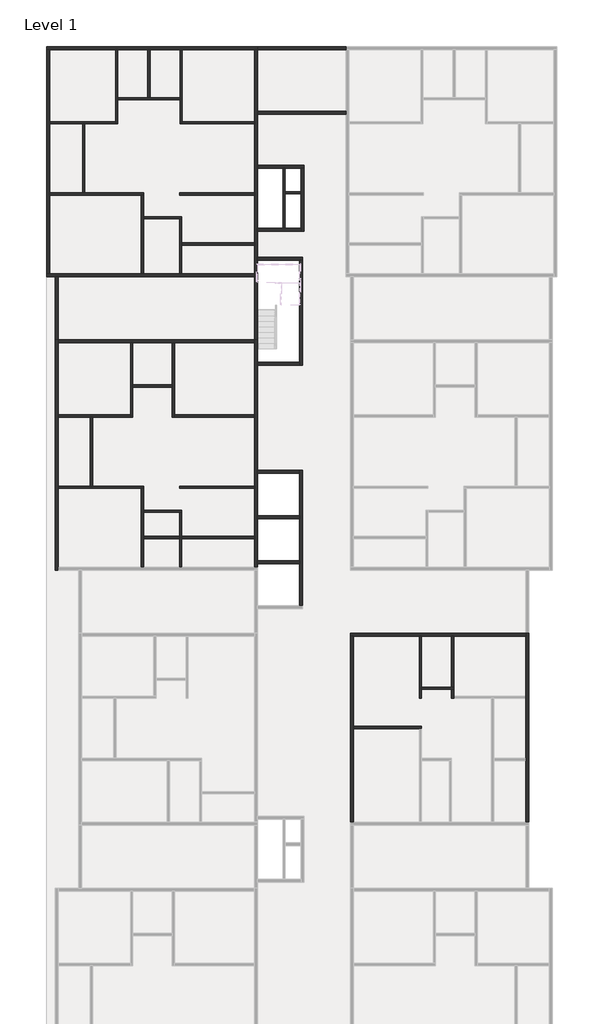
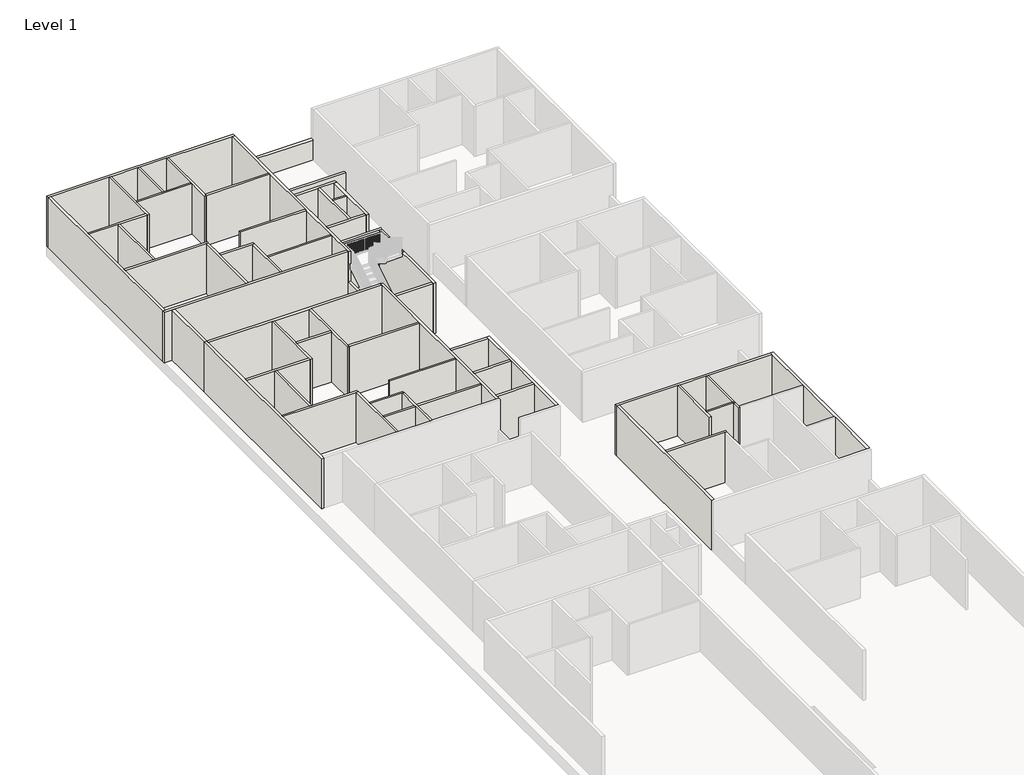
# One storey, part 3 of 8: 57 walls.
"""IFC4 building model written with IfcOpenShell, lengths in millimetres."""

from ifc_helpers import new_model, si_unit, frame, origin, place, context, project, spatial, polyline, outline, extrude, faceted_brep, element, save

model = new_model("IFC4")

# Units and contexts
model_context = context("Model", 3, world=origin())
ifc_project = project(units=[si_unit("LENGTHUNIT", "METRE", prefix="MILLI")], contexts=[model_context])

# Site, building, storey
site = spatial("IfcSite", under=ifc_project)
building = spatial("IfcBuilding", under=site)
storey = spatial("IfcBuildingStorey", under=building, Name="Level 1", Elevation=25234.6172466)

# Walls
placement = place(None, origin())
element("IfcWall", 1, ObjectType="4.5\"", at=placement, inside=storey, context=model_context, shape_type="Brep", body=[
    faceted_brep([(-10818.3415084, 35031.1216096, 25234.6172466), (-10818.3415084, 31373.5216096, 25234.6172466), (-10818.3415084, 31259.2216096, 25234.6172466), (-10818.3415084, 31259.2216096, 28282.6172466), (-10818.3415084, 31373.5216096, 28282.6172466), (-10818.3415084, 35031.1216096, 28282.6172466), (-10704.0415084, 35031.1216096, 25234.6172466), (-10704.0415084, 35031.1216096, 28282.6172466), (-10704.0415084, 32592.7216096, 28282.6172466), (-10704.0415084, 32478.4216096, 28282.6172466), (-10704.0415084, 31259.2216096, 28282.6172466), (-10704.0415084, 31259.2216096, 25234.6172466), (-10704.0415084, 32478.4216096, 25234.6172466), (-10704.0415084, 32592.7216096, 25234.6172466)], [[[0, 1, 2, 3, 4, 5]], [[6, 7, 8, 9, 10, 11, 12, 13]], [[2, 1, 0, 6, 13, 12, 11]], [[0, 5, 7, 6]], [[3, 2, 11, 10]], [[5, 4, 3, 10, 9, 8, 7]]]),
])
element("IfcWall", 2, ObjectType="4.5\"", at=placement, inside=storey, context=model_context, shape_type="Brep", body=[
    faceted_brep([(-10818.3415084, 31373.5216096, 25234.6172466), (-14171.1415084, 31373.5216096, 25234.6172466), (-14171.1415084, 31373.5216096, 28282.6172466), (-10818.3415084, 31373.5216096, 28282.6172466), (-10818.3415084, 31259.2216096, 25234.6172466), (-10818.3415084, 31259.2216096, 28282.6172466), (-12380.4415084, 31259.2216096, 28282.6172466), (-12494.7415084, 31259.2216096, 28282.6172466), (-14171.1415084, 31259.2216096, 28282.6172466), (-14171.1415084, 31259.2216096, 25234.6172466), (-12494.7415084, 31259.2216096, 25234.6172466), (-12380.4415084, 31259.2216096, 25234.6172466)], [[[0, 1, 2, 3]], [[4, 5, 6, 7, 8, 9, 10, 11]], [[1, 0, 4, 11, 10, 9]], [[0, 3, 5, 4]], [[2, 1, 9, 8]], [[3, 2, 8, 7, 6, 5]]]),
])
element("IfcWall", 3, ObjectType="4.5\"", at=placement, inside=storey, context=model_context, shape_type="SweptSolid", body=[
    extrude(outline(polyline([(-12494.7415084, 27754.0216096), (-12494.7415084, 31259.2216096), (-12380.4415084, 31259.2216096), (-12380.4415084, 27754.0216096), (-12494.7415084, 27754.0216096)])), frame((0.0, 0.0, 25234.6172466), z_axis=(0.0, 0.0, 1.0), x_axis=(1.0, 0.0, 0.0)), (0.0, 0.0, 1.0), 3048.0),
])
element("IfcWall", 4, ObjectType="4.5\"", at=placement, inside=storey, context=model_context, shape_type="Brep", body=[
    faceted_brep([(-14171.1415084, 27639.7216096, 25234.6172466), (-9510.2415084, 27639.7216096, 25234.6172466), (-9395.9415084, 27639.7216096, 25234.6172466), (-9395.9415084, 27639.7216096, 28282.6172466), (-9510.2415084, 27639.7216096, 28282.6172466), (-14171.1415084, 27639.7216096, 28282.6172466), (-14171.1415084, 27754.0216096, 25234.6172466), (-14171.1415084, 27754.0216096, 28282.6172466), (-12494.7415084, 27754.0216096, 28282.6172466), (-12380.4415084, 27754.0216096, 28282.6172466), (-9395.9415084, 27754.0216096, 28282.6172466), (-9395.9415084, 27754.0216096, 25234.6172466), (-12380.4415084, 27754.0216096, 25234.6172466), (-12494.7415084, 27754.0216096, 25234.6172466)], [[[0, 1, 2, 3, 4, 5]], [[6, 7, 8, 9, 10, 11, 12, 13]], [[2, 1, 0, 6, 13, 12, 11]], [[0, 5, 7, 6]], [[3, 2, 11, 10]], [[5, 4, 3, 10, 9, 8, 7]]]),
])
element("IfcWall", 5, ObjectType="4.5\"", at=placement, inside=storey, context=model_context, shape_type="Brep", body=[
    faceted_brep([(-9510.2415084, 27639.7216096, 25234.6172466), (-9510.2415084, 23651.9216096, 25234.6172466), (-9510.2415084, 23651.9216096, 28282.6172466), (-9510.2415084, 27639.7216096, 28282.6172466), (-9395.9415084, 27639.7216096, 25234.6172466), (-9395.9415084, 27639.7216096, 28282.6172466), (-9395.9415084, 26547.5216096, 28282.6172466), (-9395.9415084, 26433.2216096, 28282.6172466), (-9395.9415084, 23651.9216096, 28282.6172466), (-9395.9415084, 23651.9216096, 25234.6172466), (-9395.9415084, 26433.2216096, 25234.6172466), (-9395.9415084, 26547.5216096, 25234.6172466)], [[[0, 1, 2, 3]], [[4, 5, 6, 7, 8, 9, 10, 11]], [[1, 0, 4, 11, 10, 9]], [[0, 3, 5, 4]], [[2, 1, 9, 8]], [[3, 2, 8, 7, 6, 5]]]),
])
element("IfcWall", 6, ObjectType="4.5\"", at=placement, inside=storey, context=model_context, shape_type="Brep", body=[
    faceted_brep([(-9395.9415084, 26433.2216096, 25234.6172466), (-7567.1415084, 26433.2216096, 25234.6172466), (-7452.8415084, 26433.2216096, 25234.6172466), (-7452.8415084, 26433.2216096, 28282.6172466), (-7567.1415084, 26433.2216096, 28282.6172466), (-9395.9415084, 26433.2216096, 28282.6172466), (-9395.9415084, 26547.5216096, 25234.6172466), (-9395.9415084, 26547.5216096, 28282.6172466), (-7452.8415084, 26547.5216096, 28282.6172466), (-7452.8415084, 26547.5216096, 25234.6172466)], [[[0, 1, 2, 3, 4, 5]], [[6, 7, 8, 9]], [[2, 1, 0, 6, 9]], [[0, 5, 7, 6]], [[3, 2, 9, 8]], [[5, 4, 3, 8, 7]]]),
])
element("IfcWall", 7, ObjectType="4.5\"", at=placement, inside=storey, context=model_context, shape_type="Brep", body=[
    faceted_brep([(-7567.1415084, 26433.2216096, 25234.6172466), (-7567.1415084, 23651.9216096, 25234.6172466), (-7567.1415084, 23651.9216096, 28282.6172466), (-7567.1415084, 26433.2216096, 28282.6172466), (-7452.8415084, 26433.2216096, 25234.6172466), (-7452.8415084, 26433.2216096, 28282.6172466), (-7452.8415084, 25214.0216096, 28282.6172466), (-7452.8415084, 25099.7216096, 28282.6172466), (-7452.8415084, 23651.9216096, 28282.6172466), (-7452.8415084, 23651.9216096, 25234.6172466), (-7452.8415084, 25099.7216096, 25234.6172466), (-7452.8415084, 25214.0216096, 25234.6172466)], [[[0, 1, 2, 3]], [[4, 5, 6, 7, 8, 9, 10, 11]], [[1, 0, 4, 11, 10, 9]], [[0, 3, 5, 4]], [[2, 1, 9, 8]], [[3, 2, 8, 7, 6, 5]]]),
])
element("IfcWall", 8, ObjectType="4.5\"", at=placement, inside=storey, context=model_context, shape_type="SweptSolid", body=[
    extrude(outline(polyline([(-7452.8415084, 25214.0216096), (-3769.8415084, 25214.0216096), (-3769.8415084, 25099.7216096), (-7452.8415084, 25099.7216096), (-7452.8415084, 25214.0216096)])), frame((0.0, 0.0, 25234.6172466), z_axis=(0.0, 0.0, 1.0), x_axis=(1.0, 0.0, 0.0)), (0.0, 0.0, 1.0), 3048.0),
])
element("IfcWall", 9, ObjectType="4.5\"", at=placement, inside=storey, context=model_context, shape_type="SweptSolid", body=[
    extrude(outline(polyline([(-3769.8415084, 27639.7216096), (-7567.1415084, 27639.7216096), (-7567.1415084, 27754.0216096), (-3769.8415084, 27754.0216096), (-3769.8415084, 27639.7216096)])), frame((0.0, 0.0, 25234.6172466), z_axis=(0.0, 0.0, 1.0), x_axis=(1.0, 0.0, 0.0)), (0.0, 0.0, 1.0), 3048.0),
])
element("IfcWall", 10, ObjectType="4.5\"", at=placement, inside=storey, context=model_context, shape_type="Brep", body=[
    faceted_brep([(-10704.0415084, 32478.4216096, 25234.6172466), (-7541.7415084, 32478.4216096, 25234.6172466), (-7541.7415084, 32478.4216096, 28282.6172466), (-10704.0415084, 32478.4216096, 28282.6172466), (-10704.0415084, 32592.7216096, 25234.6172466), (-10704.0415084, 32592.7216096, 28282.6172466), (-9180.0415084, 32592.7216096, 28282.6172466), (-9065.7415084, 32592.7216096, 28282.6172466), (-7541.7415084, 32592.7216096, 28282.6172466), (-7541.7415084, 32592.7216096, 25234.6172466), (-9065.7415084, 32592.7216096, 25234.6172466), (-9180.0415084, 32592.7216096, 25234.6172466)], [[[0, 1, 2, 3]], [[4, 5, 6, 7, 8, 9, 10, 11]], [[1, 0, 4, 11, 10, 9]], [[0, 3, 5, 4]], [[2, 1, 9, 8]], [[3, 2, 8, 7, 6, 5]]]),
])
element("IfcWall", 11, ObjectType="4.5\"", at=placement, inside=storey, context=model_context, shape_type="SweptSolid", body=[
    extrude(outline(polyline([(-9180.0415084, 32592.7216096), (-9180.0415084, 35031.1216096), (-9065.7415084, 35031.1216096), (-9065.7415084, 32592.7216096), (-9180.0415084, 32592.7216096)])), frame((0.0, 0.0, 25234.6172466), z_axis=(0.0, 0.0, 1.0), x_axis=(1.0, 0.0, 0.0)), (0.0, 0.0, 1.0), 3048.0),
])
element("IfcWall", 12, ObjectType="4.5\"", at=placement, inside=storey, context=model_context, shape_type="Brep", body=[
    faceted_brep([(-7541.7415084, 35031.1216096, 25234.6172466), (-7541.7415084, 32592.7216096, 25234.6172466), (-7541.7415084, 32478.4216096, 25234.6172466), (-7541.7415084, 31259.2216096, 25234.6172466), (-7541.7415084, 31259.2216096, 28282.6172466), (-7541.7415084, 32478.4216096, 28282.6172466), (-7541.7415084, 32592.7216096, 28282.6172466), (-7541.7415084, 35031.1216096, 28282.6172466), (-7427.4415084, 35031.1216096, 25234.6172466), (-7427.4415084, 35031.1216096, 28282.6172466), (-7427.4415084, 31373.5216096, 28282.6172466), (-7427.4415084, 31259.2216096, 28282.6172466), (-7427.4415084, 31259.2216096, 25234.6172466), (-7427.4415084, 31373.5216096, 25234.6172466)], [[[0, 1, 2, 3, 4, 5, 6, 7]], [[8, 9, 10, 11, 12, 13]], [[3, 2, 1, 0, 8, 13, 12]], [[0, 7, 9, 8]], [[4, 3, 12, 11]], [[7, 6, 5, 4, 11, 10, 9]]]),
])
element("IfcWall", 13, ObjectType="4.5\"", at=placement, inside=storey, context=model_context, shape_type="SweptSolid", body=[
    extrude(outline(polyline([(-3769.8415084, 31259.2216096), (-7427.4415084, 31259.2216096), (-7427.4415084, 31373.5216096), (-3769.8415084, 31373.5216096), (-3769.8415084, 31259.2216096)])), frame((0.0, 0.0, 25234.6172466), z_axis=(0.0, 0.0, 1.0), x_axis=(1.0, 0.0, 0.0)), (0.0, 0.0, 1.0), 3048.0),
])
element("IfcWall", 14, ObjectType="4.5\"", at=placement, inside=storey, context=model_context, shape_type="Brep", body=[
    faceted_brep([(-10061.4044854, 20146.7216096, 25234.6172466), (-10061.4044854, 16489.1216096, 25234.6172466), (-10061.4044854, 16374.8216096, 25234.6172466), (-10061.4044854, 16374.8216096, 28282.6172466), (-10061.4044854, 16489.1216096, 28282.6172466), (-10061.4044854, 20146.7216096, 28282.6172466), (-9947.1044854, 20146.7216096, 25234.6172466), (-9947.1044854, 20146.7216096, 28282.6172466), (-9947.1044854, 18013.1216096, 28282.6172466), (-9947.1044854, 17898.8216096, 28282.6172466), (-9947.1044854, 16374.8216096, 28282.6172466), (-9947.1044854, 16374.8216096, 25234.6172466), (-9947.1044854, 17898.8216096, 25234.6172466), (-9947.1044854, 18013.1216096, 25234.6172466)], [[[0, 1, 2, 3, 4, 5]], [[6, 7, 8, 9, 10, 11, 12, 13]], [[2, 1, 0, 6, 13, 12, 11]], [[0, 5, 7, 6]], [[3, 2, 11, 10]], [[5, 4, 3, 10, 9, 8, 7]]]),
])
element("IfcWall", 15, ObjectType="4.5\"", at=placement, inside=storey, context=model_context, shape_type="Brep", body=[
    faceted_brep([(-10061.4044854, 16489.1216096, 25234.6172466), (-13719.0044854, 16489.1216096, 25234.6172466), (-13719.0044854, 16489.1216096, 28282.6172466), (-10061.4044854, 16489.1216096, 28282.6172466), (-10061.4044854, 16374.8216096, 25234.6172466), (-10061.4044854, 16374.8216096, 28282.6172466), (-11980.3915084, 16374.8216096, 28282.6172466), (-12094.6915084, 16374.8216096, 28282.6172466), (-13719.0044854, 16374.8216096, 28282.6172466), (-13719.0044854, 16374.8216096, 25234.6172466), (-12094.6915084, 16374.8216096, 25234.6172466), (-11980.3915084, 16374.8216096, 25234.6172466)], [[[0, 1, 2, 3]], [[4, 5, 6, 7, 8, 9, 10, 11]], [[1, 0, 4, 11, 10, 9]], [[0, 3, 5, 4]], [[2, 1, 9, 8]], [[3, 2, 8, 7, 6, 5]]]),
])
element("IfcWall", 16, ObjectType="4.5\"", at=placement, inside=storey, context=model_context, shape_type="SweptSolid", body=[
    extrude(outline(polyline([(-7940.5044854, 17898.8216096), (-9947.1044854, 17898.8216096), (-9947.1044854, 18013.1216096), (-7940.5044854, 18013.1216096), (-7940.5044854, 17898.8216096)])), frame((0.0, 0.0, 25234.6172466), z_axis=(0.0, 0.0, 1.0), x_axis=(1.0, 0.0, 0.0)), (0.0, 0.0, 1.0), 3048.0),
])
element("IfcWall", 17, ObjectType="4.5\"", at=placement, inside=storey, context=model_context, shape_type="Brep", body=[
    faceted_brep([(-7940.5044854, 20146.7216096, 25234.6172466), (-7940.5044854, 18013.1216096, 25234.6172466), (-7940.5044854, 17898.8216096, 25234.6172466), (-7940.5044854, 16374.8216096, 25234.6172466), (-7940.5044854, 16374.8216096, 28282.6172466), (-7940.5044854, 17898.8216096, 28282.6172466), (-7940.5044854, 18013.1216096, 28282.6172466), (-7940.5044854, 20146.7216096, 28282.6172466), (-7826.2044854, 20146.7216096, 25234.6172466), (-7826.2044854, 20146.7216096, 28282.6172466), (-7826.2044854, 16489.1216096, 28282.6172466), (-7826.2044854, 16374.8216096, 28282.6172466), (-7826.2044854, 16374.8216096, 25234.6172466), (-7826.2044854, 16489.1216096, 25234.6172466)], [[[0, 1, 2, 3, 4, 5, 6, 7]], [[8, 9, 10, 11, 12, 13]], [[3, 2, 1, 0, 8, 13, 12]], [[0, 7, 9, 8]], [[4, 3, 12, 11]], [[7, 6, 5, 4, 11, 10, 9]]]),
])
element("IfcWall", 18, ObjectType="4.5\"", at=placement, inside=storey, context=model_context, shape_type="SweptSolid", body=[
    extrude(outline(polyline([(-3769.8415084, 16374.8216096), (-7826.2044854, 16374.8216096), (-7826.2044854, 16489.1216096), (-3769.8415084, 16489.1216096), (-3769.8415084, 16374.8216096)])), frame((0.0, 0.0, 25234.6172466), z_axis=(0.0, 0.0, 1.0), x_axis=(1.0, 0.0, 0.0)), (0.0, 0.0, 1.0), 3048.0),
])
element("IfcWall", 19, ObjectType="4.5\"", at=placement, inside=storey, context=model_context, shape_type="SweptSolid", body=[
    extrude(outline(polyline([(-12094.6915084, 12869.6216096), (-12094.6915084, 16374.8216096), (-11980.3915084, 16374.8216096), (-11980.3915084, 12869.6216096), (-12094.6915084, 12869.6216096)])), frame((0.0, 0.0, 25234.6172466), z_axis=(0.0, 0.0, 1.0), x_axis=(1.0, 0.0, 0.0)), (0.0, 0.0, 1.0), 3048.0),
])
element("IfcWall", 20, ObjectType="4.5\"", at=placement, inside=storey, context=model_context, shape_type="Brep", body=[
    faceted_brep([(-13719.0044854, 12755.3216096, 25234.6172466), (-9510.2415084, 12755.3216096, 25234.6172466), (-9395.9415084, 12755.3216096, 25234.6172466), (-9395.9415084, 12755.3216096, 28282.6172466), (-9510.2415084, 12755.3216096, 28282.6172466), (-13719.0044854, 12755.3216096, 28282.6172466), (-13719.0044854, 12869.6216096, 25234.6172466), (-13719.0044854, 12869.6216096, 28282.6172466), (-12094.6915084, 12869.6216096, 28282.6172466), (-11980.3915084, 12869.6216096, 28282.6172466), (-9395.9415084, 12869.6216096, 28282.6172466), (-9395.9415084, 12869.6216096, 25234.6172466), (-11980.3915084, 12869.6216096, 25234.6172466), (-12094.6915084, 12869.6216096, 25234.6172466)], [[[0, 1, 2, 3, 4, 5]], [[6, 7, 8, 9, 10, 11, 12, 13]], [[2, 1, 0, 6, 13, 12, 11]], [[0, 5, 7, 6]], [[3, 2, 11, 10]], [[5, 4, 3, 10, 9, 8, 7]]]),
])
element("IfcWall", 21, ObjectType="4.5\"", at=placement, inside=storey, context=model_context, shape_type="Brep", body=[
    faceted_brep([(-9510.2415084, 12755.3216096, 25234.6172466), (-9510.2415084, 8767.5216096, 25234.6172466), (-9510.2415084, 8767.5216096, 28282.6172466), (-9510.2415084, 12755.3216096, 28282.6172466), (-9395.9415084, 12755.3216096, 25234.6172466), (-9395.9415084, 12755.3216096, 28282.6172466), (-9395.9415084, 11663.1216096, 28282.6172466), (-9395.9415084, 11548.8216096, 28282.6172466), (-9395.9415084, 10329.6216096, 28282.6172466), (-9395.9415084, 10215.3216096, 28282.6172466), (-9395.9415084, 8767.5216096, 28282.6172466), (-9395.9415084, 8767.5216096, 25234.6172466), (-9395.9415084, 10215.3216096, 25234.6172466), (-9395.9415084, 10329.6216096, 25234.6172466), (-9395.9415084, 11548.8216096, 25234.6172466), (-9395.9415084, 11663.1216096, 25234.6172466)], [[[0, 1, 2, 3]], [[4, 5, 6, 7, 8, 9, 10, 11, 12, 13, 14, 15]], [[1, 0, 4, 15, 14, 13, 12, 11]], [[0, 3, 5, 4]], [[2, 1, 11, 10]], [[3, 2, 10, 9, 8, 7, 6, 5]]]),
])
element("IfcWall", 22, ObjectType="4.5\"", at=placement, inside=storey, context=model_context, shape_type="SweptSolid", body=[
    extrude(outline(polyline([(-7567.1415084, 10215.3216096), (-9395.9415084, 10215.3216096), (-9395.9415084, 10329.6216096), (-7567.1415084, 10329.6216096), (-7567.1415084, 10215.3216096)])), frame((0.0, 0.0, 25234.6172466), z_axis=(0.0, 0.0, 1.0), x_axis=(1.0, 0.0, 0.0)), (0.0, 0.0, 1.0), 3048.0),
])
element("IfcWall", 23, ObjectType="4.5\"", at=placement, inside=storey, context=model_context, shape_type="Brep", body=[
    faceted_brep([(-9395.9415084, 11548.8216096, 25234.6172466), (-7567.1415084, 11548.8216096, 25234.6172466), (-7452.8415084, 11548.8216096, 25234.6172466), (-7452.8415084, 11548.8216096, 28282.6172466), (-7567.1415084, 11548.8216096, 28282.6172466), (-9395.9415084, 11548.8216096, 28282.6172466), (-9395.9415084, 11663.1216096, 25234.6172466), (-9395.9415084, 11663.1216096, 28282.6172466), (-7452.8415084, 11663.1216096, 28282.6172466), (-7452.8415084, 11663.1216096, 25234.6172466)], [[[0, 1, 2, 3, 4, 5]], [[6, 7, 8, 9]], [[2, 1, 0, 6, 9]], [[0, 5, 7, 6]], [[3, 2, 9, 8]], [[5, 4, 3, 8, 7]]]),
])
element("IfcWall", 24, ObjectType="4.5\"", at=placement, inside=storey, context=model_context, shape_type="Brep", body=[
    faceted_brep([(-7567.1415084, 11548.8216096, 25234.6172466), (-7567.1415084, 10329.6216096, 25234.6172466), (-7567.1415084, 10215.3216096, 25234.6172466), (-7567.1415084, 8767.5216096, 25234.6172466), (-7567.1415084, 8767.5216096, 28282.6172466), (-7567.1415084, 10215.3216096, 28282.6172466), (-7567.1415084, 10329.6216096, 28282.6172466), (-7567.1415084, 11548.8216096, 28282.6172466), (-7452.8415084, 11548.8216096, 25234.6172466), (-7452.8415084, 11548.8216096, 28282.6172466), (-7452.8415084, 10329.6216096, 28282.6172466), (-7452.8415084, 10215.3216096, 28282.6172466), (-7452.8415084, 8767.5216096, 28282.6172466), (-7452.8415084, 8767.5216096, 25234.6172466), (-7452.8415084, 10215.3216096, 25234.6172466), (-7452.8415084, 10329.6216096, 25234.6172466)], [[[0, 1, 2, 3, 4, 5, 6, 7]], [[8, 9, 10, 11, 12, 13, 14, 15]], [[3, 2, 1, 0, 8, 15, 14, 13]], [[0, 7, 9, 8]], [[4, 3, 13, 12]], [[7, 6, 5, 4, 12, 11, 10, 9]]]),
])
element("IfcWall", 25, ObjectType="4.5\"", at=placement, inside=storey, context=model_context, shape_type="SweptSolid", body=[
    extrude(outline(polyline([(-3769.8415084, 10215.3216096), (-7452.8415084, 10215.3216096), (-7452.8415084, 10329.6216096), (-3769.8415084, 10329.6216096), (-3769.8415084, 10215.3216096)])), frame((0.0, 0.0, 25234.6172466), z_axis=(0.0, 0.0, 1.0), x_axis=(1.0, 0.0, 0.0)), (0.0, 0.0, 1.0), 3048.0),
])
element("IfcWall", 26, ObjectType="4.5\"", at=placement, inside=storey, context=model_context, shape_type="SweptSolid", body=[
    extrude(outline(polyline([(-3769.8415084, 12755.3216096), (-7567.1415084, 12755.3216096), (-7567.1415084, 12869.6216096), (-3769.8415084, 12869.6216096), (-3769.8415084, 12755.3216096)])), frame((0.0, 0.0, 25234.6172466), z_axis=(0.0, 0.0, 1.0), x_axis=(1.0, 0.0, 0.0)), (0.0, 0.0, 1.0), 3048.0),
])
element("IfcWall", 27, ObjectType="4.5\"", at=placement, inside=storey, context=model_context, shape_type="Brep", body=[
    faceted_brep([(1259.3584916, 572.7745083, 25234.6172466), (4610.8714687, 572.7745083, 25234.6172466), (4725.1714687, 572.7745083, 25234.6172466), (4725.1714687, 572.7745083, 28282.6172466), (4610.8714687, 572.7745083, 28282.6172466), (1259.3584916, 572.7745083, 28282.6172466), (1259.3584916, 687.0745083, 25234.6172466), (1259.3584916, 687.0745083, 28282.6172466), (4725.1714687, 687.0745083, 28282.6172466), (4725.1714687, 687.0745083, 25234.6172466)], [[[0, 1, 2, 3, 4, 5]], [[6, 7, 8, 9]], [[2, 1, 0, 6, 9]], [[0, 5, 7, 6]], [[3, 2, 9, 8]], [[5, 4, 3, 8, 7]]]),
])
element("IfcWall", 28, ObjectType="4.5\"", at=placement, inside=storey, context=model_context, shape_type="Brep", body=[
    faceted_brep([(4610.8714687, 5262.3216096, 25234.6172466), (4610.8714687, 2100.0216096, 25234.6172466), (4610.8714687, 2100.0216096, 28282.6172466), (4610.8714687, 5262.3216096, 28282.6172466), (4725.1714687, 5262.3216096, 25234.6172466), (4725.1714687, 5262.3216096, 28282.6172466), (4725.1714687, 2671.5216096, 28282.6172466), (4725.1714687, 2557.2216096, 28282.6172466), (4725.1714687, 2100.0216096, 28282.6172466), (4725.1714687, 2100.0216096, 25234.6172466), (4725.1714687, 2557.2216096, 25234.6172466), (4725.1714687, 2671.5216096, 25234.6172466)], [[[0, 1, 2, 3]], [[4, 5, 6, 7, 8, 9, 10, 11]], [[1, 0, 4, 11, 10, 9]], [[2, 1, 9, 8]], [[0, 3, 5, 4]], [[3, 2, 8, 7, 6, 5]]]),
])
element("IfcWall", 29, ObjectType="4.5\"", at=placement, inside=storey, context=model_context, shape_type="Brep", body=[
    faceted_brep([(4725.1714687, 2557.2216096, 25234.6172466), (6249.1714687, 2557.2216096, 25234.6172466), (6363.4714687, 2557.2216096, 25234.6172466), (6363.4714687, 2557.2216096, 28282.6172466), (6249.1714687, 2557.2216096, 28282.6172466), (4725.1714687, 2557.2216096, 28282.6172466), (4725.1714687, 2671.5216096, 25234.6172466), (4725.1714687, 2671.5216096, 28282.6172466), (6249.1714687, 2671.5216096, 28282.6172466), (6363.4714687, 2671.5216096, 28282.6172466), (6363.4714687, 2671.5216096, 25234.6172466), (6249.1714687, 2671.5216096, 25234.6172466)], [[[0, 1, 2, 3, 4, 5]], [[6, 7, 8, 9, 10, 11]], [[2, 1, 0, 6, 11, 10]], [[0, 5, 7, 6]], [[3, 2, 10, 9]], [[5, 4, 3, 9, 8, 7]]]),
])
element("IfcWall", 30, ObjectType="4.5\"", at=placement, inside=storey, context=model_context, shape_type="SweptSolid", body=[
    extrude(outline(polyline([(6363.4714687, 5262.3216096), (6363.4714687, 2671.5216096), (6249.1714687, 2671.5216096), (6249.1714687, 5262.3216096), (6363.4714687, 5262.3216096)])), frame((0.0, 0.0, 25234.6172466), z_axis=(0.0, 0.0, 1.0), x_axis=(1.0, 0.0, 0.0)), (0.0, 0.0, 1.0), 3048.0),
])
element("IfcWall", 31, ObjectType="4.5\"", at=placement, inside=storey, context=model_context, shape_type="Brep", body=[
    faceted_brep([(6249.1714687, 2557.2216096, 25234.6172466), (6249.1714687, 2100.0216096, 25234.6172466), (6249.1714687, 2100.0216096, 28282.6172466), (6249.1714687, 2557.2216096, 28282.6172466), (6363.4714687, 2557.2216096, 25234.6172466), (6363.4714687, 2557.2216096, 28282.6172466), (6363.4714687, 2214.3216096, 28282.6172466), (6363.4714687, 2100.0216096, 28282.6172466), (6363.4714687, 2100.0216096, 25234.6172466), (6363.4714687, 2214.3216096, 25234.6172466)], [[[0, 1, 2, 3]], [[4, 5, 6, 7, 8, 9]], [[1, 0, 4, 9, 8]], [[0, 3, 5, 4]], [[2, 1, 8, 7]], [[3, 2, 7, 6, 5]]]),
])
element("IfcWall", 32, ObjectType="4.5\"", at=placement, inside=storey, context=model_context, shape_type="Brep", body=[
    faceted_brep([(-2321.9738684, 29000.0900967, 25234.6172466), (-2321.9738684, 25952.0900967, 25234.6172466), (-2321.9738684, 25952.0900967, 28282.6172466), (-2321.9738684, 29000.0900967, 28282.6172466), (-2207.6738684, 29000.0900967, 25234.6172466), (-2207.6738684, 29000.0900967, 28282.6172466), (-2207.6738684, 27820.8172885, 28282.6172466), (-2207.6738684, 27706.5172885, 28282.6172466), (-2207.6738684, 25952.0900967, 28282.6172466), (-2207.6738684, 25952.0900967, 25234.6172466), (-2207.6738684, 27706.5172885, 25234.6172466), (-2207.6738684, 27820.8172885, 25234.6172466)], [[[0, 1, 2, 3]], [[4, 5, 6, 7, 8, 9, 10, 11]], [[1, 0, 4, 11, 10, 9]], [[3, 2, 8, 7, 6, 5]], [[0, 3, 5, 4]], [[2, 1, 9, 8]]]),
])
element("IfcWall", 33, ObjectType="4.5\"", at=placement, inside=storey, context=model_context, shape_type="SweptSolid", body=[
    extrude(outline(polyline([(-2207.6738684, 27820.8172885), (-1407.6415084, 27820.8172885), (-1407.6415084, 27706.5172885), (-2207.6738684, 27706.5172885), (-2207.6738684, 27820.8172885)])), frame((0.0, 0.0, 25234.6172466), z_axis=(0.0, 0.0, 1.0), x_axis=(1.0, 0.0, 0.0)), (0.0, 0.0, 1.0), 3048.0),
])
element("IfcWall", 34, ObjectType="6\"", at=placement, inside=storey, context=model_context, shape_type="Brep", body=[
    faceted_brep([(-14323.5415084, 35031.1216096, 25234.6172466), (-14171.1415084, 35031.1216096, 25234.6172466), (-10818.3415084, 35031.1216096, 25234.6172466), (-10704.0415084, 35031.1216096, 25234.6172466), (-9180.0415084, 35031.1216096, 25234.6172466), (-9065.7415084, 35031.1216096, 25234.6172466), (-7541.7415084, 35031.1216096, 25234.6172466), (-7427.4415084, 35031.1216096, 25234.6172466), (-3769.8415084, 35031.1216096, 25234.6172466), (-3617.4415084, 35031.1216096, 25234.6172466), (-3617.4415084, 35031.1216096, 28282.6172466), (-3769.8415084, 35031.1216096, 28282.6172466), (-7427.4415084, 35031.1216096, 28282.6172466), (-7541.7415084, 35031.1216096, 28282.6172466), (-9065.7415084, 35031.1216096, 28282.6172466), (-9180.0415084, 35031.1216096, 28282.6172466), (-10704.0415084, 35031.1216096, 28282.6172466), (-10818.3415084, 35031.1216096, 28282.6172466), (-14171.1415084, 35031.1216096, 28282.6172466), (-14323.5415084, 35031.1216096, 28282.6172466), (-14323.5415084, 35183.5216096, 25234.6172466), (-14323.5415084, 35183.5216096, 28282.6172466), (-3617.4415084, 35183.5216096, 28282.6172466), (-3617.4415084, 35183.5216096, 25234.6172466)], [[[0, 1, 2, 3, 4, 5, 6, 7, 8, 9, 10, 11, 12, 13, 14, 15, 16, 17, 18, 19]], [[20, 21, 22, 23]], [[9, 8, 7, 6, 5, 4, 3, 2, 1, 0, 20, 23]], [[0, 19, 21, 20]], [[9, 23, 22, 10]], [[19, 18, 17, 16, 15, 14, 13, 12, 11, 10, 22, 21]]]),
])
element("IfcWall", 35, ObjectType="6\"", at=placement, inside=storey, context=model_context, shape_type="Brep", body=[
    faceted_brep([(-3769.8415084, 35031.1216096, 28282.6172466), (-3769.8415084, 35031.1216096, 25234.6172466), (-3769.8415084, 31373.5216096, 25234.6172466), (-3769.8415084, 31259.2216096, 25234.6172466), (-3769.8415084, 27754.0216096, 25234.6172466), (-3769.8415084, 27639.7216096, 25234.6172466), (-3769.8415084, 25214.0216096, 25234.6172466), (-3769.8415084, 25099.7216096, 25234.6172466), (-3769.8415084, 23651.9216096, 25234.6172466), (-3769.8415084, 23499.5216096, 25234.6172466), (-3769.8415084, 23499.5216096, 28282.6172466), (-3769.8415084, 23651.9216096, 28282.6172466), (-3769.8415084, 25099.7216096, 28282.6172466), (-3769.8415084, 25214.0216096, 28282.6172466), (-3769.8415084, 27639.7216096, 28282.6172466), (-3769.8415084, 27754.0216096, 28282.6172466), (-3769.8415084, 31259.2216096, 28282.6172466), (-3769.8415084, 31373.5216096, 28282.6172466), (-3617.4415084, 35031.1216096, 25234.6172466), (-3617.4415084, 35031.1216096, 28282.6172466), (-3617.4415084, 29152.4900967, 28282.6172466), (-3617.4415084, 29000.0900967, 28282.6172466), (-3617.4415084, 25952.0900967, 28282.6172466), (-3617.4415084, 25799.6900967, 28282.6172466), (-3617.4415084, 24490.1216096, 28282.6172466), (-3617.4415084, 24337.7216096, 28282.6172466), (-3617.4415084, 23499.5216096, 28282.6172466), (-3617.4415084, 23499.5216096, 25234.6172466), (-3617.4415084, 24337.7216096, 25234.6172466), (-3617.4415084, 24490.1216096, 25234.6172466), (-3617.4415084, 25799.6900967, 25234.6172466), (-3617.4415084, 25952.0900967, 25234.6172466), (-3617.4415084, 29000.0900967, 25234.6172466), (-3617.4415084, 29152.4900967, 25234.6172466), (-3617.4415084, 31744.9197155, 25234.6172466), (-3617.4415084, 31897.3197155, 25234.6172466)], [[[0, 1, 2, 3, 4, 5, 6, 7, 8, 9, 10, 11, 12, 13, 14, 15, 16, 17]], [[18, 19, 20, 21, 22, 23, 24, 25, 26, 27, 28, 29, 30, 31, 32, 33, 34, 35]], [[9, 8, 7, 6, 5, 4, 3, 2, 1, 18, 35, 34, 33, 32, 31, 30, 29, 28, 27]], [[0, 19, 18, 1]], [[9, 27, 26, 10]], [[0, 17, 16, 15, 14, 13, 12, 11, 10, 26, 25, 24, 23, 22, 21, 20, 19]]]),
])
element("IfcWall", 36, ObjectType="6\"", at=placement, inside=storey, context=model_context, shape_type="Brep", body=[
    faceted_brep([(-3769.8415084, 23651.9216096, 28282.6172466), (-3769.8415084, 23651.9216096, 25234.6172466), (-7452.8415084, 23651.9216096, 25234.6172466), (-7567.1415084, 23651.9216096, 25234.6172466), (-9395.9415084, 23651.9216096, 25234.6172466), (-9510.2415084, 23651.9216096, 25234.6172466), (-14171.1415084, 23651.9216096, 25234.6172466), (-14323.5415084, 23651.9216096, 25234.6172466), (-14323.5415084, 23651.9216096, 28282.6172466), (-14171.1415084, 23651.9216096, 28282.6172466), (-9510.2415084, 23651.9216096, 28282.6172466), (-9395.9415084, 23651.9216096, 28282.6172466), (-7567.1415084, 23651.9216096, 28282.6172466), (-7452.8415084, 23651.9216096, 28282.6172466), (-3769.8415084, 23499.5216096, 25234.6172466), (-3769.8415084, 23499.5216096, 28282.6172466), (-13719.0044854, 23499.5216096, 28282.6172466), (-13871.4044854, 23499.5216096, 28282.6172466), (-14323.5415084, 23499.5216096, 28282.6172466), (-14323.5415084, 23499.5216096, 25234.6172466), (-13871.4044854, 23499.5216096, 25234.6172466), (-13719.0044854, 23499.5216096, 25234.6172466)], [[[0, 1, 2, 3, 4, 5, 6, 7, 8, 9, 10, 11, 12, 13]], [[14, 15, 16, 17, 18, 19, 20, 21]], [[7, 6, 5, 4, 3, 2, 1, 14, 21, 20, 19]], [[8, 7, 19, 18]], [[0, 15, 14, 1]], [[0, 13, 12, 11, 10, 9, 8, 18, 17, 16, 15]]]),
])
element("IfcWall", 37, ObjectType="6\"", at=placement, inside=storey, context=model_context, shape_type="Brep", body=[
    faceted_brep([(-14171.1415084, 23651.9216096, 25234.6172466), (-14171.1415084, 27639.7216096, 25234.6172466), (-14171.1415084, 27754.0216096, 25234.6172466), (-14171.1415084, 31259.2216096, 25234.6172466), (-14171.1415084, 31373.5216096, 25234.6172466), (-14171.1415084, 35031.1216096, 25234.6172466), (-14171.1415084, 35031.1216096, 28282.6172466), (-14171.1415084, 31373.5216096, 28282.6172466), (-14171.1415084, 31259.2216096, 28282.6172466), (-14171.1415084, 27754.0216096, 28282.6172466), (-14171.1415084, 27639.7216096, 28282.6172466), (-14171.1415084, 23651.9216096, 28282.6172466), (-14323.5415084, 23651.9216096, 25234.6172466), (-14323.5415084, 23651.9216096, 28282.6172466), (-14323.5415084, 35031.1216096, 28282.6172466), (-14323.5415084, 35031.1216096, 25234.6172466)], [[[0, 1, 2, 3, 4, 5, 6, 7, 8, 9, 10, 11]], [[12, 13, 14, 15]], [[5, 4, 3, 2, 1, 0, 12, 15]], [[6, 5, 15, 14]], [[0, 11, 13, 12]], [[11, 10, 9, 8, 7, 6, 14, 13]]]),
])
element("IfcWall", 38, ObjectType="6\"", at=placement, inside=storey, context=model_context, shape_type="Brep", body=[
    faceted_brep([(-13871.4044854, 20299.1216096, 25234.6172466), (-13871.4044854, 8615.1216096, 25234.6172466), (-13871.4044854, 8615.1216096, 28282.6172466), (-13871.4044854, 20299.1216096, 28282.6172466), (-13719.0044854, 20299.1216096, 25234.6172466), (-13719.0044854, 20299.1216096, 28282.6172466), (-13719.0044854, 20146.7216096, 28282.6172466), (-13719.0044854, 16489.1216096, 28282.6172466), (-13719.0044854, 16374.8216096, 28282.6172466), (-13719.0044854, 12869.6216096, 28282.6172466), (-13719.0044854, 12755.3216096, 28282.6172466), (-13719.0044854, 8767.5216096, 28282.6172466), (-13719.0044854, 8615.1216096, 28282.6172466), (-13719.0044854, 8615.1216096, 25234.6172466), (-13719.0044854, 8767.5216096, 25234.6172466), (-13719.0044854, 12755.3216096, 25234.6172466), (-13719.0044854, 12869.6216096, 25234.6172466), (-13719.0044854, 16374.8216096, 25234.6172466), (-13719.0044854, 16489.1216096, 25234.6172466), (-13719.0044854, 20146.7216096, 25234.6172466)], [[[0, 1, 2, 3]], [[4, 5, 6, 7, 8, 9, 10, 11, 12, 13, 14, 15, 16, 17, 18, 19]], [[1, 0, 4, 19, 18, 17, 16, 15, 14, 13]], [[2, 1, 13, 12]], [[0, 3, 5, 4]], [[3, 2, 12, 11, 10, 9, 8, 7, 6, 5]]]),
])
element("IfcWall", 39, ObjectType="6\"", at=placement, inside=storey, context=model_context, shape_type="Brep", body=[
    faceted_brep([(-3617.4415084, 8767.5216096, 28282.6172466), (-3617.4415084, 8767.5216096, 25234.6172466), (-3617.4415084, 8945.2303368, 25234.6172466), (-3617.4415084, 9097.6303368, 25234.6172466), (-3617.4415084, 11231.2303368, 25234.6172466), (-3617.4415084, 11383.6303368, 25234.6172466), (-3617.4415084, 13517.2303368, 25234.6172466), (-3617.4415084, 13669.6303368, 25234.6172466), (-3617.4415084, 19003.7216096, 25234.6172466), (-3617.4415084, 19156.1216096, 25234.6172466), (-3617.4415084, 20299.1216096, 25234.6172466), (-3617.4415084, 20299.1216096, 28282.6172466), (-3617.4415084, 19156.1216096, 28282.6172466), (-3617.4415084, 19003.7216096, 28282.6172466), (-3617.4415084, 13669.6303368, 28282.6172466), (-3617.4415084, 13517.2303368, 28282.6172466), (-3617.4415084, 11383.6303368, 28282.6172466), (-3617.4415084, 11231.2303368, 28282.6172466), (-3617.4415084, 9097.6303368, 28282.6172466), (-3617.4415084, 8945.2303368, 28282.6172466), (-3769.8415084, 8767.5216096, 25234.6172466), (-3769.8415084, 8767.5216096, 28282.6172466), (-3769.8415084, 10215.3216096, 28282.6172466), (-3769.8415084, 10329.6216096, 28282.6172466), (-3769.8415084, 12755.3216096, 28282.6172466), (-3769.8415084, 12869.6216096, 28282.6172466), (-3769.8415084, 16374.8216096, 28282.6172466), (-3769.8415084, 16489.1216096, 28282.6172466), (-3769.8415084, 20146.7216096, 28282.6172466), (-3769.8415084, 20299.1216096, 28282.6172466), (-3769.8415084, 20299.1216096, 25234.6172466), (-3769.8415084, 20146.7216096, 25234.6172466), (-3769.8415084, 16489.1216096, 25234.6172466), (-3769.8415084, 16374.8216096, 25234.6172466), (-3769.8415084, 12869.6216096, 25234.6172466), (-3769.8415084, 12755.3216096, 25234.6172466), (-3769.8415084, 10329.6216096, 25234.6172466), (-3769.8415084, 10215.3216096, 25234.6172466)], [[[0, 1, 2, 3, 4, 5, 6, 7, 8, 9, 10, 11, 12, 13, 14, 15, 16, 17, 18, 19]], [[20, 21, 22, 23, 24, 25, 26, 27, 28, 29, 30, 31, 32, 33, 34, 35, 36, 37]], [[10, 9, 8, 7, 6, 5, 4, 3, 2, 1, 20, 37, 36, 35, 34, 33, 32, 31, 30]], [[10, 30, 29, 11]], [[0, 21, 20, 1]], [[0, 19, 18, 17, 16, 15, 14, 13, 12, 11, 29, 28, 27, 26, 25, 24, 23, 22, 21]]]),
])
element("IfcWall", 40, ObjectType="6\"", at=placement, inside=storey, context=model_context, shape_type="Brep", body=[
    faceted_brep([(-3769.8415084, 20299.1216096, 28282.6172466), (-3769.8415084, 20299.1216096, 25234.6172466), (-13719.0044854, 20299.1216096, 25234.6172466), (-13719.0044854, 20299.1216096, 28282.6172466), (-3769.8415084, 20146.7216096, 25234.6172466), (-3769.8415084, 20146.7216096, 28282.6172466), (-7826.2044854, 20146.7216096, 28282.6172466), (-7940.5044854, 20146.7216096, 28282.6172466), (-9947.1044854, 20146.7216096, 28282.6172466), (-10061.4044854, 20146.7216096, 28282.6172466), (-13719.0044854, 20146.7216096, 28282.6172466), (-13719.0044854, 20146.7216096, 25234.6172466), (-10061.4044854, 20146.7216096, 25234.6172466), (-9947.1044854, 20146.7216096, 25234.6172466), (-7940.5044854, 20146.7216096, 25234.6172466), (-7826.2044854, 20146.7216096, 25234.6172466)], [[[0, 1, 2, 3]], [[4, 5, 6, 7, 8, 9, 10, 11, 12, 13, 14, 15]], [[2, 1, 4, 15, 14, 13, 12, 11]], [[3, 2, 11, 10]], [[0, 5, 4, 1]], [[0, 3, 10, 9, 8, 7, 6, 5]]]),
])
element("IfcWall", 41, ObjectType="6\"", at=placement, inside=storey, context=model_context, shape_type="Brep", body=[
    faceted_brep([(10173.4714687, -4185.9344126, 28282.6172466), (10173.4714687, -4185.9344126, 25234.6172466), (10173.4714687, 5414.7216096, 25234.6172466), (10173.4714687, 5414.7216096, 28282.6172466), (10021.0714687, -4185.9344126, 25234.6172466), (10021.0714687, -4185.9344126, 28282.6172466), (10021.0714687, -1061.7344126, 28282.6172466), (10021.0714687, -947.4344126, 28282.6172466), (10021.0714687, 2100.0216096, 28282.6172466), (10021.0714687, 2214.3216096, 28282.6172466), (10021.0714687, 5262.3216096, 28282.6172466), (10021.0714687, 5414.7216096, 28282.6172466), (10021.0714687, 5414.7216096, 25234.6172466), (10021.0714687, 5262.3216096, 25234.6172466), (10021.0714687, 2214.3216096, 25234.6172466), (10021.0714687, 2100.0216096, 25234.6172466), (10021.0714687, -947.4344126, 25234.6172466), (10021.0714687, -1061.7344126, 25234.6172466)], [[[0, 1, 2, 3]], [[4, 5, 6, 7, 8, 9, 10, 11, 12, 13, 14, 15, 16, 17]], [[2, 1, 4, 17, 16, 15, 14, 13, 12]], [[2, 12, 11, 3]], [[0, 5, 4, 1]], [[0, 3, 11, 10, 9, 8, 7, 6, 5]]]),
])
element("IfcWall", 42, ObjectType="6\"", at=placement, inside=storey, context=model_context, shape_type="Brep", body=[
    faceted_brep([(10021.0714687, 5414.7216096, 28282.6172466), (10021.0714687, 5414.7216096, 25234.6172466), (1106.9584916, 5414.7216096, 25234.6172466), (1106.9584916, 5414.7216096, 28282.6172466), (10021.0714687, 5262.3216096, 25234.6172466), (10021.0714687, 5262.3216096, 28282.6172466), (6363.4714687, 5262.3216096, 28282.6172466), (6249.1714687, 5262.3216096, 28282.6172466), (4725.1714687, 5262.3216096, 28282.6172466), (4610.8714687, 5262.3216096, 28282.6172466), (1259.3584916, 5262.3216096, 28282.6172466), (1106.9584916, 5262.3216096, 28282.6172466), (1106.9584916, 5262.3216096, 25234.6172466), (1259.3584916, 5262.3216096, 25234.6172466), (4610.8714687, 5262.3216096, 25234.6172466), (4725.1714687, 5262.3216096, 25234.6172466), (6249.1714687, 5262.3216096, 25234.6172466), (6363.4714687, 5262.3216096, 25234.6172466)], [[[0, 1, 2, 3]], [[4, 5, 6, 7, 8, 9, 10, 11, 12, 13, 14, 15, 16, 17]], [[2, 1, 4, 17, 16, 15, 14, 13, 12]], [[3, 2, 12, 11]], [[0, 5, 4, 1]], [[0, 3, 11, 10, 9, 8, 7, 6, 5]]]),
])
element("IfcWall", 43, ObjectType="6\"", at=placement, inside=storey, context=model_context, shape_type="Brep", body=[
    faceted_brep([(1106.9584916, 5262.3216096, 25234.6172466), (1106.9584916, -4185.9344126, 25234.6172466), (1106.9584916, -4185.9344126, 28282.6172466), (1106.9584916, 5262.3216096, 28282.6172466), (1259.3584916, 5262.3216096, 25234.6172466), (1259.3584916, 5262.3216096, 28282.6172466), (1259.3584916, 687.0745083, 28282.6172466), (1259.3584916, 572.7745083, 28282.6172466), (1259.3584916, -4185.9344126, 28282.6172466), (1259.3584916, -4185.9344126, 25234.6172466), (1259.3584916, 572.7745083, 25234.6172466), (1259.3584916, 687.0745083, 25234.6172466)], [[[0, 1, 2, 3]], [[4, 5, 6, 7, 8, 9, 10, 11]], [[1, 0, 4, 11, 10, 9]], [[0, 3, 5, 4]], [[1, 9, 8, 2]], [[3, 2, 8, 7, 6, 5]]]),
])
element("IfcWall", 44, ObjectType="6\"", at=placement, inside=storey, context=model_context, shape_type="Brep", body=[
    faceted_brep([(-1331.4415084, 6811.6303368, 25234.6172466), (-1331.4415084, 13669.6303368, 25234.6172466), (-1331.4415084, 13669.6303368, 28282.6172466), (-1331.4415084, 6811.6303368, 28282.6172466), (-1483.8415084, 6811.6303368, 25234.6172466), (-1483.8415084, 6811.6303368, 28282.6172466), (-1483.8415084, 8945.2303368, 28282.6172466), (-1483.8415084, 9097.6303368, 28282.6172466), (-1483.8415084, 11231.2303368, 28282.6172466), (-1483.8415084, 11383.6303368, 28282.6172466), (-1483.8415084, 13517.2303368, 28282.6172466), (-1483.8415084, 13669.6303368, 28282.6172466), (-1483.8415084, 13669.6303368, 25234.6172466), (-1483.8415084, 13517.2303368, 25234.6172466), (-1483.8415084, 11383.6303368, 25234.6172466), (-1483.8415084, 11231.2303368, 25234.6172466), (-1483.8415084, 9097.6303368, 25234.6172466), (-1483.8415084, 8945.2303368, 25234.6172466)], [[[0, 1, 2, 3]], [[4, 5, 6, 7, 8, 9, 10, 11, 12, 13, 14, 15, 16, 17]], [[1, 0, 4, 17, 16, 15, 14, 13, 12]], [[3, 2, 11, 10, 9, 8, 7, 6, 5]], [[0, 3, 5, 4]], [[2, 1, 12, 11]]]),
])
element("IfcWall", 45, ObjectType="6\"", at=placement, inside=storey, context=model_context, shape_type="SweptSolid", body=[
    extrude(outline(polyline([(-3617.4415084, 13669.6303368), (-1483.8415084, 13669.6303368), (-1483.8415084, 13517.2303368), (-3617.4415084, 13517.2303368), (-3617.4415084, 13669.6303368)])), frame((0.0, 0.0, 25234.6172466), z_axis=(0.0, 0.0, 1.0), x_axis=(1.0, 0.0, 0.0)), (0.0, 0.0, 1.0), 3048.0),
])
element("IfcWall", 46, ObjectType="6\"", at=placement, inside=storey, context=model_context, shape_type="SweptSolid", body=[
    extrude(outline(polyline([(-1483.8415084, 8945.2303368), (-3617.4415084, 8945.2303368), (-3617.4415084, 9097.6303368), (-1483.8415084, 9097.6303368), (-1483.8415084, 8945.2303368)])), frame((0.0, 0.0, 25234.6172466), z_axis=(0.0, 0.0, 1.0), x_axis=(1.0, 0.0, 0.0)), (0.0, 0.0, 1.0), 3048.0),
])
element("IfcWall", 47, ObjectType="6\"", at=placement, inside=storey, context=model_context, shape_type="SweptSolid", body=[
    extrude(outline(polyline([(-3617.4415084, 11383.6303368), (-1483.8415084, 11383.6303368), (-1483.8415084, 11231.2303368), (-3617.4415084, 11231.2303368), (-3617.4415084, 11383.6303368)])), frame((0.0, 0.0, 25234.6172466), z_axis=(0.0, 0.0, 1.0), x_axis=(1.0, 0.0, 0.0)), (0.0, 0.0, 1.0), 3048.0),
])
element("IfcWall", 48, ObjectType="6\"", at=placement, inside=storey, context=model_context, shape_type="Brep", body=[
    faceted_brep([(-3617.4415084, 29000.0900967, 25234.6172466), (-2321.9738684, 29000.0900967, 25234.6172466), (-2207.6738684, 29000.0900967, 25234.6172466), (-1407.6415084, 29000.0900967, 25234.6172466), (-1255.2415084, 29000.0900967, 25234.6172466), (-1255.2415084, 29000.0900967, 28282.6172466), (-1407.6415084, 29000.0900967, 28282.6172466), (-2207.6738684, 29000.0900967, 28282.6172466), (-2321.9738684, 29000.0900967, 28282.6172466), (-3617.4415084, 29000.0900967, 28282.6172466), (-3617.4415084, 29152.4900967, 25234.6172466), (-3617.4415084, 29152.4900967, 28282.6172466), (-1255.2415084, 29152.4900967, 28282.6172466), (-1255.2415084, 29152.4900967, 25234.6172466)], [[[0, 1, 2, 3, 4, 5, 6, 7, 8, 9]], [[10, 11, 12, 13]], [[4, 3, 2, 1, 0, 10, 13]], [[9, 8, 7, 6, 5, 12, 11]], [[0, 9, 11, 10]], [[5, 4, 13, 12]]]),
])
element("IfcWall", 49, ObjectType="6\"", at=placement, inside=storey, context=model_context, shape_type="Brep", body=[
    faceted_brep([(-1407.6415084, 29000.0900967, 25234.6172466), (-1407.6415084, 27820.8172885, 25234.6172466), (-1407.6415084, 27706.5172885, 25234.6172466), (-1407.6415084, 25952.0900967, 25234.6172466), (-1407.6415084, 25799.6900967, 25234.6172466), (-1407.6415084, 25799.6900967, 28282.6172466), (-1407.6415084, 25952.0900967, 28282.6172466), (-1407.6415084, 27706.5172885, 28282.6172466), (-1407.6415084, 27820.8172885, 28282.6172466), (-1407.6415084, 29000.0900967, 28282.6172466), (-1255.2415084, 29000.0900967, 25234.6172466), (-1255.2415084, 29000.0900967, 28282.6172466), (-1255.2415084, 25799.6900967, 28282.6172466), (-1255.2415084, 25799.6900967, 25234.6172466)], [[[0, 1, 2, 3, 4, 5, 6, 7, 8, 9]], [[10, 11, 12, 13]], [[4, 3, 2, 1, 0, 10, 13]], [[9, 8, 7, 6, 5, 12, 11]], [[0, 9, 11, 10]], [[5, 4, 13, 12]]]),
])
element("IfcWall", 50, ObjectType="6\"", at=placement, inside=storey, context=model_context, shape_type="Brep", body=[
    faceted_brep([(-1407.6415084, 25952.0900967, 25234.6172466), (-2207.6738684, 25952.0900967, 25234.6172466), (-2321.9738684, 25952.0900967, 25234.6172466), (-3617.4415084, 25952.0900967, 25234.6172466), (-3617.4415084, 25952.0900967, 28282.6172466), (-2321.9738684, 25952.0900967, 28282.6172466), (-2207.6738684, 25952.0900967, 28282.6172466), (-1407.6415084, 25952.0900967, 28282.6172466), (-1407.6415084, 25799.6900967, 25234.6172466), (-1407.6415084, 25799.6900967, 28282.6172466), (-3617.4415084, 25799.6900967, 28282.6172466), (-3617.4415084, 25799.6900967, 25234.6172466)], [[[0, 1, 2, 3, 4, 5, 6, 7]], [[8, 9, 10, 11]], [[3, 2, 1, 0, 8, 11]], [[7, 6, 5, 4, 10, 9]], [[0, 7, 9, 8]], [[4, 3, 11, 10]]]),
])
element("IfcWall", 51, ObjectType="6\"", at=placement, inside=storey, context=model_context, shape_type="Brep", body=[
    faceted_brep([(-3617.4415084, 24337.7216096, 25234.6172466), (-1483.8415084, 24337.7216096, 25234.6172466), (-1331.4415084, 24337.7216096, 25234.6172466), (-1331.4415084, 24337.7216096, 28282.6172466), (-1483.8415084, 24337.7216096, 28282.6172466), (-3617.4415084, 24337.7216096, 28282.6172466), (-3617.4415084, 24490.1216096, 25234.6172466), (-3617.4415084, 24490.1216096, 28282.6172466), (-1331.4415084, 24490.1216096, 28282.6172466), (-1331.4415084, 24490.1216096, 25234.6172466)], [[[0, 1, 2, 3, 4, 5]], [[6, 7, 8, 9]], [[2, 1, 0, 6, 9]], [[5, 4, 3, 8, 7]], [[0, 5, 7, 6]], [[3, 2, 9, 8]]]),
])
element("IfcWall", 52, ObjectType="6\"", at=placement, inside=storey, context=model_context, shape_type="Brep", body=[
    faceted_brep([(-1483.8415084, 24337.7216096, 25234.6172466), (-1483.8415084, 19156.1216096, 25234.6172466), (-1483.8415084, 19003.7216096, 25234.6172466), (-1483.8415084, 19003.7216096, 28282.6172466), (-1483.8415084, 19156.1216096, 28282.6172466), (-1483.8415084, 24337.7216096, 28282.6172466), (-1331.4415084, 24337.7216096, 25234.6172466), (-1331.4415084, 24337.7216096, 28282.6172466), (-1331.4415084, 19003.7216096, 28282.6172466), (-1331.4415084, 19003.7216096, 25234.6172466)], [[[0, 1, 2, 3, 4, 5]], [[6, 7, 8, 9]], [[2, 1, 0, 6, 9]], [[5, 4, 3, 8, 7]], [[0, 5, 7, 6]], [[3, 2, 9, 8]]]),
])
element("IfcWall", 53, ObjectType="6\"", at=placement, inside=storey, context=model_context, shape_type="SweptSolid", body=[
    extrude(outline(polyline([(-3617.4415084, 19156.1216096), (-1483.8415084, 19156.1216096), (-1483.8415084, 19003.7216096), (-3617.4415084, 19003.7216096), (-3617.4415084, 19156.1216096)])), frame((0.0, 0.0, 25234.6172466), z_axis=(0.0, 0.0, 1.0), x_axis=(1.0, 0.0, 0.0)), (0.0, 0.0, 1.0), 3048.0),
])
element("IfcWall", 54, ObjectType="6\" 2", at=placement, inside=storey, context=model_context, shape_type="SweptSolid", body=[
    extrude(outline(polyline([(-13871.4044854, 20299.1216096), (-13871.4044854, 23499.5216096), (-13719.0044854, 23499.5216096), (-13719.0044854, 20299.1216096), (-13871.4044854, 20299.1216096)])), frame((0.0, 0.0, 25234.6172466), z_axis=(0.0, 0.0, 1.0), x_axis=(1.0, 0.0, 0.0)), (0.0, 0.0, 1.0), 3048.0),
])
element("IfcWall", 55, ObjectType="6\" 2", at=placement, inside=storey, context=model_context, shape_type="SweptSolid", body=[
    extrude(outline(polyline([(878.4443719, 35031.1216096), (-3617.4415084, 35031.1216096), (-3617.4415084, 35183.5216096), (878.4443719, 35183.5216096), (878.4443719, 35031.1216096)])), frame((0.0, 0.0, 25234.6172466), z_axis=(0.0, 0.0, 1.0), x_axis=(1.0, 0.0, 0.0)), (0.0, 0.0, 1.0), 1219.2),
])
element("IfcWall", 56, ObjectType="6\" 2", at=placement, inside=storey, context=model_context, shape_type="SweptSolid", body=[
    extrude(outline(polyline([(878.4443719, 31744.9197155), (-3617.4415084, 31744.9197155), (-3617.4415084, 31897.3197155), (878.4443719, 31897.3197155), (878.4443719, 31744.9197155)])), frame((0.0, 0.0, 25234.6172466), z_axis=(0.0, 0.0, 1.0), x_axis=(1.0, 0.0, 0.0)), (0.0, 0.0, 1.0), 1219.2),
])
element("IfcWall", 57, ObjectType="6\" 2", at=placement, inside=storey, context=model_context, shape_type="SweptSolid", body=[
    extrude(outline(polyline([(-3769.8415084, 20299.1216096), (-3769.8415084, 23499.5216096), (-3617.4415084, 23499.5216096), (-3617.4415084, 20299.1216096), (-3769.8415084, 20299.1216096)])), frame((0.0, 0.0, 25234.6172466), z_axis=(0.0, 0.0, 1.0), x_axis=(1.0, 0.0, 0.0)), (0.0, 0.0, 1.0), 1219.2),
])

save(model, "model.ifc")

# Revit data of these elements
# Type "4.5\""
#   Assembly Code = "B2010"
#   Layers, outside or top first: 0' - 4 1/2" "WALLS" (function 1)
# Type "6\""
#   Assembly Code = "B2010"
#   Layers, outside or top first: 0' - 6" "WALLS" (function 1)
# Type "6\" 2"
#   Assembly Code = "B2010"
#   Layers, outside or top first: 0' - 6" "4'" (function 1)
# Elements 1, 2, 3, 4, 5, 6, 7, 8, 9, 10, 11, 12, 13, 14, 15, 16, 17, 18, 19, 20, 21, 22, 23, 24, 25, 26, 27, 28, 29, 30, 31, 32, 33 (IfcWall, "4.5\"")
#   Top Offset = 0' - 0"
#   Base Offset = 0' - 0"
#   Unconnected Height = 10' - 0"
#   wall height = 10' - 0"
#   Phase Created = New Construction
#   Base Constraint = Level 1
#   Materials on its faces: "WALLS"
# Elements 34, 35, 36, 37, 38, 39, 40, 41, 42, 43, 44, 45, 46, 47, 48, 49, 50, 51, 52, 53 (IfcWall, "6\"")
#   Top Offset = 0' - 0"
#   Base Offset = 0' - 0"
#   Unconnected Height = 10' - 0"
#   wall height = 10' - 0"
#   Phase Created = New Construction
#   Base Constraint = Level 1
#   Materials on its faces: "WALLS"
# Element 54 (IfcWall, "6\" 2")
#   Top Offset = 0' - 0"
#   Base Offset = 0' - 0"
#   Unconnected Height = 10' - 0"
#   wall height = 10' - 0"
#   Phase Created = New Construction
#   Base Constraint = Level 1
#   Materials on its faces: "4'"
# Elements 55, 56, 57 (IfcWall, "6\" 2")
#   Top Offset = 0' - 0"
#   Base Offset = 0' - 0"
#   Unconnected Height = 4' - 0"
#   wall height = 4' - 0"
#   Phase Created = New Construction
#   Base Constraint = Level 1
#   Materials on its faces: "4'"
# Materials
#   "WALLS": class "Generic", colour RGB 120 120 120, transparency 0, Cost = 0
#   "4'": class "Generic", colour RGB 120 120 120, transparency 0, Cost = 0
